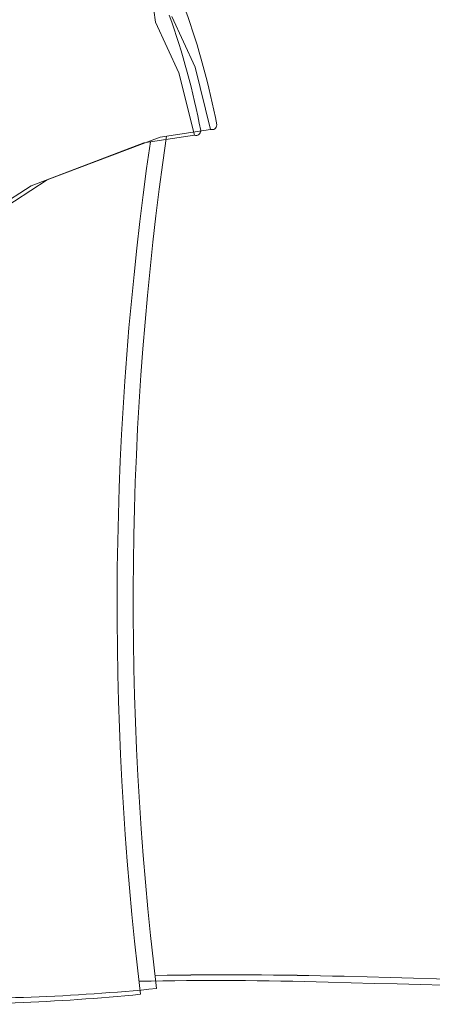
# Model space of a CAD drawing. Units: inches. Extents: x 1885 to 2748, y 783 to 2421.
# Tile 10 of 117: x 2001 to 2017, y 1139 to 1178. Entities that reach past the tile are written whole.
import ezdxf

# ---------------------------------------------------------------- set-up
doc = ezdxf.new("R2010")
doc.units = ezdxf.units.IN
doc.layers.add('A-FURN', color=8, linetype='Continuous', lineweight=13)

# ---------------------------------------------------------------- blocks, each defined once
blk = doc.blocks.new('BED-DOUBLE')
for p, q in [((28.833, 40.953), (28.369, 44.36)), ((28.833, 40.952), (28.369, 44.36)), ((30.401, 39.168), (29.472, 41.181)), ((30.401, 39.167), (29.472, 41.181)), ((29.762, 38.939), (28.833, 40.953)), ((29.762, 38.939), (28.833, 40.952)), ((30.381, 36.461), (29.762, 38.939)), ((30.381, 36.461), (29.762, 38.939)), ((31.02, 36.69), (30.401, 39.168)), ((31.02, 36.689), (30.401, 39.167)), ((28.369, 36.152), (30.381, 36.461)), ((28.369, 36.151), (30.381, 36.461)), ((29.008, 36.38), (31.02, 36.69)), ((29.008, 36.38), (31.02, 36.689)), ((23.88, 34.448), (28.369, 36.152)), ((23.88, 34.448), (28.369, 36.151)), ((24.519, 34.676), (29.008, 36.38)), ((24.519, 34.676), (29.008, 36.38)), ((18.026, 30.486), (24.519, 34.676)), ((18.026, 30.486), (24.519, 34.676)), ((17.387, 30.258), (23.88, 34.448)), ((17.387, 30.258), (23.88, 34.448))]:
    blk.add_line(p, q)
for centre, radius, start, end in [((1.486, 31.152), 29.654, 10.6617, 19.8806), ((1.486, 31.152), 29.654, 10.6617, 19.8806), ((2.125, 31.381), 29.654, 10.6617, 19.8806), ((2.125, 31.381), 29.654, 10.6617, 19.8806), ((31.082, 36.863), 0.185, 250.2464, 1.1377), ((31.082, 36.863), 0.185, 250.2464, 1.1377), ((30.443, 36.635), 0.185, 250.2464, 1.1377), ((30.443, 36.635), 0.185, 250.2464, 1.1377), ((156.32, 17.754), 129.02, 171.78449, 186.90062), ((156.32, 17.754), 129.02, 171.78449, 186.90062), ((156.959, 17.983), 129.02, 171.78449, 186.90062), ((156.959, 17.983), 129.02, 171.78449, 186.90062), ((31.177, -167.309), 170.11, 88.4762, 91.00819), ((31.177, -167.309), 170.11, 88.4762, 91.00819), ((31.817, -167.08), 170.11, 88.4762, 91.00819), ((31.817, -167.081), 170.11, 88.4762, 91.00819), ((51.257, 485.049), 482.31, 268.22771, 271.71854), ((51.257, 485.049), 482.31, 268.22771, 271.71854), ((20.739, 85.389), 83.306, 268.72178, 275.60397), ((20.739, 85.389), 83.306, 268.72178, 275.60397), ((50.617, 484.821), 482.31, 268.22771, 271.71854), ((50.617, 484.821), 482.31, 268.22771, 271.71854), ((20.1, 85.16), 83.306, 268.72178, 275.60397), ((20.1, 85.16), 83.306, 268.72178, 275.60397)]:
    blk.add_arc(centre, radius, start, end)

msp = doc.modelspace()

# ---------------------------------------------------------------- block references
at = {"layer": 'A-FURN'}
msp.add_blockref('BED-DOUBLE', (1977.555, 1137.199), dxfattribs=at)

doc.saveas('drawing.dxf')
